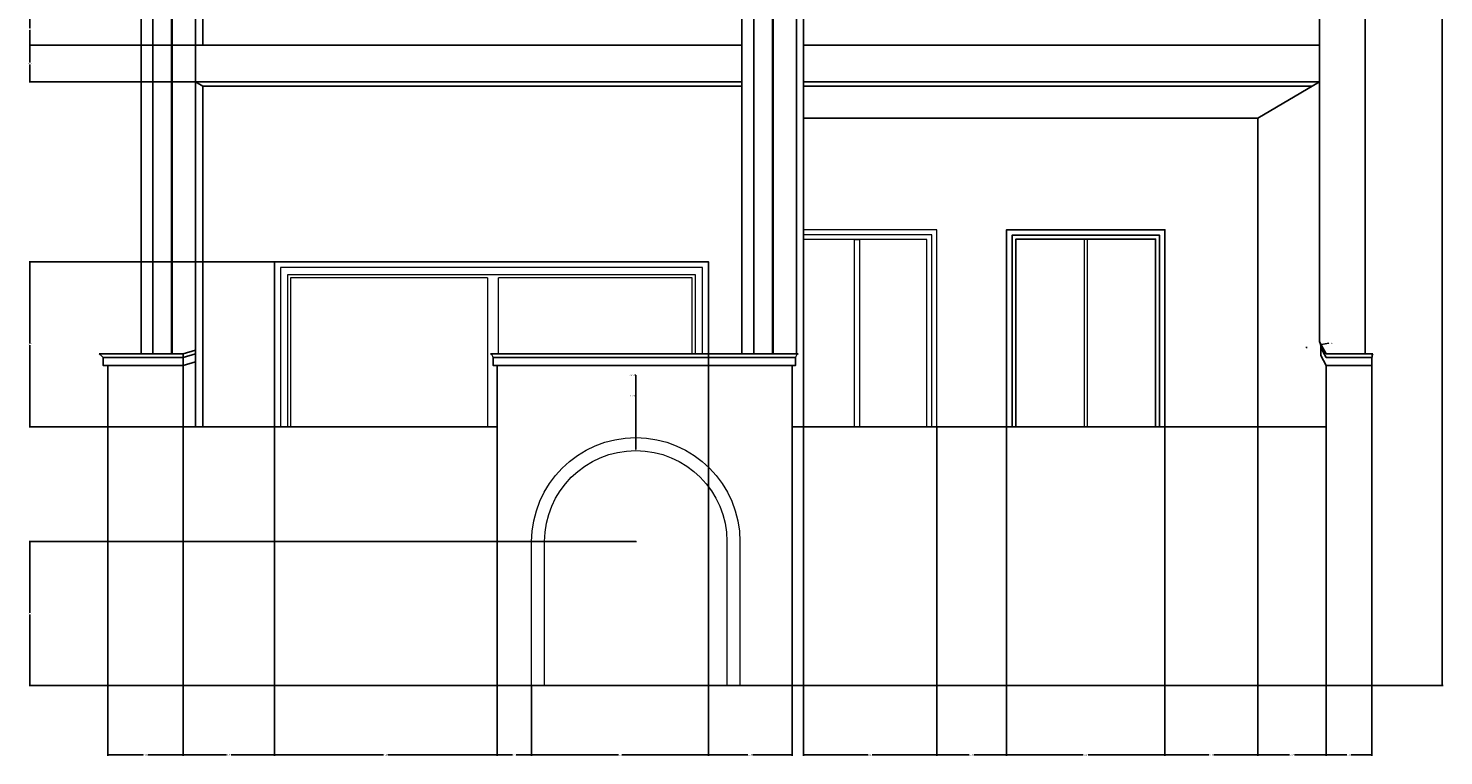
# Model space of a CAD drawing. Units: feet. Extents: x 2352 to 2983, y 950 to 1233.
# Tile 4 of 5: x 2718 to 2983, y 950 to 1086. Entities that reach past the tile are written whole.
import ezdxf

# ---------------------------------------------------------------- set-up
doc = ezdxf.new("R2010")
doc.units = ezdxf.units.FT
for name, color, linetype, lineweight in [('A-ANNO-DIMS', 2, 'Continuous', 18), ('A-DOOR', 3, 'Continuous', 18), ('A-ELEV', 7, 'Continuous', 25), ('A-GLAZ', 4, 'Continuous', 18)]:
    doc.layers.add(name, color=color, linetype=linetype, lineweight=lineweight)
doc.styles.get("Standard").update_dxf_attribs({"font": 'arial.ttf'})
doc.dimstyles.get("Standard").update_dxf_attribs({"dimtxt": 0.18, "dimasz": 0.18, "dimexe": 0.18, "dimexo": 0.0625, "dimgap": 0.09, "dimtad": 0, "dimtih": 1, "dimtoh": 1, "dimdec": 1, "dimzin": 0, "dimdsep": 46, "dimlunit": 3, "dimtxsty": 'Standard', "dimcen": 0.09, "dimadec": 0, "dimazin": 0, "dimtfac": 1, "dimtdec": 1, "dimtofl": 0, "dimtmove": 0, "dimatfit": 3, "dimfxl": 1, "dimtolj": 1, "dimtzin": 0, "dimarcsym": 0})

# ---------------------------------------------------------------- blocks, each defined once
blk = doc.blocks.new('*D30')
at = {"layer": 'A-ANNO-DIMS', "color": 0, "lineweight": -2, "transparency": 16777216}
for p, q in [((2934.99, 1219.82), (2982.56, 1219.82)), ((2982.38, 1219.64), (2982.38, 1091.6)), ((2982.38, 963.19), (2982.38, 1091.23)), ((2969.32, 963.01), (2982.56, 963.01))]:
    blk.add_line(p, q, dxfattribs=at)
at = {"layer": 'A-ANNO-DIMS', "color": 0, "transparency": 16777216}
for points in [[(2982.35, 1219.64), (2982.41, 1219.64), (2982.38, 1219.82)], [(2982.35, 963.19), (2982.41, 963.19), (2982.38, 963.01)]]:
    blk.add_solid(points, dxfattribs=at)
at = {"layer": 'Defpoints', "color": 0, "transparency": 16777216}
for p in [(2934.93, 1219.82), (2982.38, 1219.82), (2969.25, 963.01)]:
    blk.add_point(p, dxfattribs=at)
at = {"layer": 'A-ANNO-DIMS', "color": 0, "transparency": 16777216, "insert": (2982.38, 1091.42), "char_height": 0.18, "attachment_point": 5}
blk.add_mtext('\\A1;256.8', dxfattribs=at)
blk = doc.blocks.new('*D31')
at = {"layer": 'A-ANNO-DIMS', "color": 0, "lineweight": -2, "transparency": 16777216}
for p, q in [((2732.56, 962.95), (2732.56, 949.88)), ((2746.64, 962.95), (2746.64, 949.88)), ((2732.74, 950.06), (2739.15, 950.06)), ((2746.46, 950.06), (2740.06, 950.06))]:
    blk.add_line(p, q, dxfattribs=at)
at = {"layer": 'A-ANNO-DIMS', "color": 0, "transparency": 16777216}
for points in [[(2732.74, 950.09), (2732.74, 950.03), (2732.56, 950.06)], [(2746.46, 950.09), (2746.46, 950.03), (2746.64, 950.06)]]:
    blk.add_solid(points, dxfattribs=at)
at = {"layer": 'Defpoints', "color": 0, "transparency": 16777216}
for p in [(2732.56, 963.01), (2746.64, 963.01), (2746.64, 950.06)]:
    blk.add_point(p, dxfattribs=at)
at = {"layer": 'A-ANNO-DIMS', "color": 0, "transparency": 16777216, "insert": (2739.6, 950.06), "char_height": 0.18, "attachment_point": 5}
blk.add_mtext('\\A1;14.086', dxfattribs=at)
blk = doc.blocks.new('*D32')
at = {"layer": 'A-ANNO-DIMS', "color": 0, "lineweight": -2, "transparency": 16777216}
for p, q in [((2763.74, 1011.42), (2763.74, 949.88)), ((2746.64, 962.95), (2746.64, 949.88)), ((2746.82, 950.06), (2754.74, 950.06)), ((2763.56, 950.06), (2755.65, 950.06))]:
    blk.add_line(p, q, dxfattribs=at)
at = {"layer": 'A-ANNO-DIMS', "color": 0, "transparency": 16777216}
for points in [[(2746.82, 950.09), (2746.82, 950.03), (2746.64, 950.06)], [(2763.56, 950.09), (2763.56, 950.03), (2763.74, 950.06)]]:
    blk.add_solid(points, dxfattribs=at)
at = {"layer": 'Defpoints', "color": 0, "transparency": 16777216}
for p in [(2763.74, 1011.48), (2746.64, 963.01), (2763.74, 950.06)]:
    blk.add_point(p, dxfattribs=at)
at = {"layer": 'A-ANNO-DIMS', "color": 0, "transparency": 16777216, "insert": (2755.19, 950.06), "char_height": 0.18, "attachment_point": 5}
blk.add_mtext('\\A1;17.097', dxfattribs=at)
blk = doc.blocks.new('*D33')
at = {"layer": 'A-ANNO-DIMS', "color": 0, "lineweight": -2, "transparency": 16777216}
for p, q in [((2763.74, 1011.42), (2763.74, 949.88)), ((2805.43, 962.95), (2805.43, 949.88)), ((2763.92, 950.06), (2784.19, 950.06)), ((2805.25, 950.06), (2784.98, 950.06))]:
    blk.add_line(p, q, dxfattribs=at)
at = {"layer": 'A-ANNO-DIMS', "color": 0, "transparency": 16777216}
for points in [[(2763.92, 950.09), (2763.92, 950.03), (2763.74, 950.06)], [(2805.25, 950.09), (2805.25, 950.03), (2805.43, 950.06)]]:
    blk.add_solid(points, dxfattribs=at)
at = {"layer": 'Defpoints', "color": 0, "transparency": 16777216}
for p in [(2763.74, 1011.48), (2805.43, 963.01), (2805.43, 950.06)]:
    blk.add_point(p, dxfattribs=at)
at = {"layer": 'A-ANNO-DIMS', "color": 0, "transparency": 16777216, "insert": (2784.59, 950.06), "char_height": 0.18, "attachment_point": 5}
blk.add_mtext('\\A1;41.69', dxfattribs=at)
blk = doc.blocks.new('*D34')
at = {"layer": 'A-ANNO-DIMS', "color": 0, "lineweight": -2, "transparency": 16777216}
for p, q in [((2805.43, 962.95), (2805.43, 949.88)), ((2811.91, 962.95), (2811.91, 949.88)), ((2805.61, 950.06), (2808.35, 950.06)), ((2811.73, 950.06), (2809, 950.06))]:
    blk.add_line(p, q, dxfattribs=at)
at = {"layer": 'A-ANNO-DIMS', "color": 0, "transparency": 16777216}
for points in [[(2805.61, 950.09), (2805.61, 950.03), (2805.43, 950.06)], [(2811.73, 950.09), (2811.73, 950.03), (2811.91, 950.06)]]:
    blk.add_solid(points, dxfattribs=at)
at = {"layer": 'Defpoints', "color": 0, "transparency": 16777216}
for p in [(2805.43, 963.01), (2811.91, 963.01), (2811.91, 950.06)]:
    blk.add_point(p, dxfattribs=at)
at = {"layer": 'A-ANNO-DIMS', "color": 0, "transparency": 16777216, "insert": (2808.67, 950.06), "char_height": 0.18, "attachment_point": 5}
blk.add_mtext('\\A1;6.48', dxfattribs=at)
blk = doc.blocks.new('*D35')
at = {"layer": 'A-ANNO-DIMS', "color": 0, "lineweight": -2, "transparency": 16777216}
for p, q in [((2845.01, 1042.39), (2845.01, 949.88)), ((2811.91, 962.95), (2811.91, 949.88)), ((2812.09, 950.06), (2828.16, 950.06)), ((2844.83, 950.06), (2828.77, 950.06))]:
    blk.add_line(p, q, dxfattribs=at)
at = {"layer": 'A-ANNO-DIMS', "color": 0, "transparency": 16777216}
for points in [[(2812.09, 950.09), (2812.09, 950.03), (2811.91, 950.06)], [(2844.83, 950.09), (2844.83, 950.03), (2845.01, 950.06)]]:
    blk.add_solid(points, dxfattribs=at)
at = {"layer": 'Defpoints', "color": 0, "transparency": 16777216}
for p in [(2845.01, 1042.45), (2811.91, 963.01), (2845.01, 950.06)]:
    blk.add_point(p, dxfattribs=at)
at = {"layer": 'A-ANNO-DIMS', "color": 0, "transparency": 16777216, "insert": (2828.46, 950.06), "char_height": 0.18, "attachment_point": 5}
blk.add_mtext('\\A1;33.1', dxfattribs=at)
blk = doc.blocks.new('*D36')
at = {"layer": 'A-ANNO-DIMS', "color": 0, "lineweight": -2, "transparency": 16777216}
for p, q in [((2845.01, 1042.39), (2845.01, 949.88)), ((2860.71, 962.95), (2860.71, 949.88)), ((2845.19, 950.06), (2852.41, 950.06)), ((2860.53, 950.06), (2853.32, 950.06))]:
    blk.add_line(p, q, dxfattribs=at)
at = {"layer": 'A-ANNO-DIMS', "color": 0, "transparency": 16777216}
for points in [[(2845.19, 950.09), (2845.19, 950.03), (2845.01, 950.06)], [(2860.53, 950.09), (2860.53, 950.03), (2860.71, 950.06)]]:
    blk.add_solid(points, dxfattribs=at)
at = {"layer": 'Defpoints', "color": 0, "transparency": 16777216}
for p in [(2845.01, 1042.45), (2860.71, 963.01), (2860.71, 950.06)]:
    blk.add_point(p, dxfattribs=at)
at = {"layer": 'A-ANNO-DIMS', "color": 0, "transparency": 16777216, "insert": (2852.86, 950.06), "char_height": 0.18, "attachment_point": 5}
blk.add_mtext('\\A1;15.698', dxfattribs=at)
blk = doc.blocks.new('*D37')
at = {"layer": 'A-ANNO-DIMS', "color": 0, "lineweight": -2, "transparency": 16777216}
for p, q in [((2862.83, 1011.42), (2862.83, 949.88)), ((2887.78, 1011.42), (2887.78, 949.88)), ((2863.01, 950.06), (2874.91, 950.06)), ((2887.6, 950.06), (2875.7, 950.06))]:
    blk.add_line(p, q, dxfattribs=at)
at = {"layer": 'A-ANNO-DIMS', "color": 0, "transparency": 16777216}
for points in [[(2863.01, 950.09), (2863.01, 950.03), (2862.83, 950.06)], [(2887.6, 950.09), (2887.6, 950.03), (2887.78, 950.06)]]:
    blk.add_solid(points, dxfattribs=at)
at = {"layer": 'Defpoints', "color": 0, "transparency": 16777216}
for p in [(2862.83, 1011.48), (2887.78, 1011.48), (2887.78, 950.06)]:
    blk.add_point(p, dxfattribs=at)
at = {"layer": 'A-ANNO-DIMS', "color": 0, "transparency": 16777216, "insert": (2875.3, 950.06), "char_height": 0.18, "attachment_point": 5}
blk.add_mtext('\\A1;24.95', dxfattribs=at)
blk = doc.blocks.new('*D38')
at = {"layer": 'A-ANNO-DIMS', "color": 0, "lineweight": -2, "transparency": 16777216}
for p, q in [((2887.78, 1011.42), (2887.78, 949.88)), ((2900.84, 1011.42), (2900.84, 949.88)), ((2887.96, 950.06), (2893.85, 950.06)), ((2900.66, 950.06), (2894.76, 950.06))]:
    blk.add_line(p, q, dxfattribs=at)
at = {"layer": 'A-ANNO-DIMS', "color": 0, "transparency": 16777216}
for points in [[(2887.96, 950.09), (2887.96, 950.03), (2887.78, 950.06)], [(2900.66, 950.09), (2900.66, 950.03), (2900.84, 950.06)]]:
    blk.add_solid(points, dxfattribs=at)
at = {"layer": 'Defpoints', "color": 0, "transparency": 16777216}
for p in [(2887.78, 1011.48), (2900.84, 1011.48), (2900.84, 950.06)]:
    blk.add_point(p, dxfattribs=at)
at = {"layer": 'A-ANNO-DIMS', "color": 0, "transparency": 16777216, "insert": (2894.31, 950.06), "char_height": 0.18, "attachment_point": 5}
blk.add_mtext('\\A1;13.062', dxfattribs=at)
blk = doc.blocks.new('*D39')
at = {"layer": 'A-ANNO-DIMS', "color": 0, "lineweight": -2, "transparency": 16777216}
for p, q in [((2900.84, 1011.42), (2900.84, 949.88)), ((2930.49, 1011.42), (2930.49, 949.88)), ((2901.02, 950.06), (2915.2, 950.06)), ((2930.31, 950.06), (2916.13, 950.06))]:
    blk.add_line(p, q, dxfattribs=at)
at = {"layer": 'A-ANNO-DIMS', "color": 0, "transparency": 16777216}
for points in [[(2901.02, 950.09), (2901.02, 950.03), (2900.84, 950.06)], [(2930.31, 950.09), (2930.31, 950.03), (2930.49, 950.06)]]:
    blk.add_solid(points, dxfattribs=at)
at = {"layer": 'Defpoints', "color": 0, "transparency": 16777216}
for p in [(2900.84, 1011.48), (2930.49, 1011.48), (2930.49, 950.06)]:
    blk.add_point(p, dxfattribs=at)
at = {"layer": 'A-ANNO-DIMS', "color": 0, "transparency": 16777216, "insert": (2915.67, 950.06), "char_height": 0.18, "attachment_point": 5}
blk.add_mtext('\\A1;29.654', dxfattribs=at)
blk = doc.blocks.new('*D40')
at = {"layer": 'A-ANNO-DIMS', "color": 0, "lineweight": -2, "transparency": 16777216}
for p, q in [((2930.49, 1011.42), (2930.49, 949.88)), ((2947.9, 1011.42), (2947.9, 949.88)), ((2930.67, 950.06), (2938.74, 950.06)), ((2947.72, 950.06), (2939.65, 950.06))]:
    blk.add_line(p, q, dxfattribs=at)
at = {"layer": 'A-ANNO-DIMS', "color": 0, "transparency": 16777216}
for points in [[(2930.67, 950.09), (2930.67, 950.03), (2930.49, 950.06)], [(2947.72, 950.09), (2947.72, 950.03), (2947.9, 950.06)]]:
    blk.add_solid(points, dxfattribs=at)
at = {"layer": 'Defpoints', "color": 0, "transparency": 16777216}
for p in [(2930.49, 1011.48), (2947.9, 1011.48), (2947.9, 950.06)]:
    blk.add_point(p, dxfattribs=at)
at = {"layer": 'A-ANNO-DIMS', "color": 0, "transparency": 16777216, "insert": (2939.19, 950.06), "char_height": 0.18, "attachment_point": 5}
blk.add_mtext('\\A1;17.403', dxfattribs=at)
blk = doc.blocks.new('*D41')
at = {"layer": 'A-ANNO-DIMS', "color": 0, "lineweight": -2, "transparency": 16777216}
for p, q in [((2947.9, 1011.42), (2947.9, 949.88)), ((2960.69, 962.95), (2960.69, 949.88)), ((2948.08, 950.06), (2953.84, 950.06)), ((2960.51, 950.06), (2954.75, 950.06))]:
    blk.add_line(p, q, dxfattribs=at)
at = {"layer": 'A-ANNO-DIMS', "color": 0, "transparency": 16777216}
for points in [[(2948.08, 950.09), (2948.08, 950.03), (2947.9, 950.06)], [(2960.51, 950.09), (2960.51, 950.03), (2960.69, 950.06)]]:
    blk.add_solid(points, dxfattribs=at)
at = {"layer": 'Defpoints', "color": 0, "transparency": 16777216}
for p in [(2947.9, 1011.48), (2960.69, 963.01), (2960.69, 950.06)]:
    blk.add_point(p, dxfattribs=at)
at = {"layer": 'A-ANNO-DIMS', "color": 0, "transparency": 16777216, "insert": (2954.29, 950.06), "char_height": 0.18, "attachment_point": 5}
blk.add_mtext('\\A1;12.797', dxfattribs=at)
blk = doc.blocks.new('*D42')
at = {"layer": 'A-ANNO-DIMS', "color": 0, "lineweight": -2, "transparency": 16777216}
for p, q in [((2960.69, 962.95), (2960.69, 949.88)), ((2969.25, 962.95), (2969.25, 949.88)), ((2960.87, 950.06), (2964.58, 950.06)), ((2969.07, 950.06), (2965.37, 950.06))]:
    blk.add_line(p, q, dxfattribs=at)
at = {"layer": 'A-ANNO-DIMS', "color": 0, "transparency": 16777216}
for points in [[(2960.87, 950.09), (2960.87, 950.03), (2960.69, 950.06)], [(2969.07, 950.09), (2969.07, 950.03), (2969.25, 950.06)]]:
    blk.add_solid(points, dxfattribs=at)
at = {"layer": 'Defpoints', "color": 0, "transparency": 16777216}
for p in [(2960.69, 963.01), (2969.25, 963.01), (2969.25, 950.06)]:
    blk.add_point(p, dxfattribs=at)
at = {"layer": 'A-ANNO-DIMS', "color": 0, "transparency": 16777216, "insert": (2964.97, 950.06), "char_height": 0.18, "attachment_point": 5}
blk.add_mtext('\\A1;8.562', dxfattribs=at)
blk = doc.blocks.new('*D53')
at = {"layer": 'A-ANNO-DIMS', "color": 0, "lineweight": -2, "transparency": 16777216}
for p, q in [((2831.35, 989.99), (2717.79, 989.99)), ((2717.97, 989.81), (2717.97, 976.68)), ((2717.97, 963.19), (2717.97, 976.32)), ((2850.84, 963.01), (2717.79, 963.01))]:
    blk.add_line(p, q, dxfattribs=at)
at = {"layer": 'A-ANNO-DIMS', "color": 0, "transparency": 16777216}
for points in [[(2717.94, 989.81), (2718, 989.81), (2717.97, 989.99)], [(2717.94, 963.19), (2718, 963.19), (2717.97, 963.01)]]:
    blk.add_solid(points, dxfattribs=at)
at = {"layer": 'Defpoints', "color": 0, "transparency": 16777216}
for p in [(2717.97, 989.99), (2831.41, 989.99), (2850.91, 963.01)]:
    blk.add_point(p, dxfattribs=at)
at = {"layer": 'A-ANNO-DIMS', "color": 0, "transparency": 16777216, "insert": (2717.97, 976.5), "char_height": 0.18, "attachment_point": 5}
blk.add_mtext('\\A1;26.98', dxfattribs=at)
blk = doc.blocks.new('*D54')
at = {"layer": 'A-ANNO-DIMS', "color": 0, "lineweight": -2, "transparency": 16777216}
for p, q in [((2763.68, 1042.45), (2717.79, 1042.45)), ((2717.97, 1042.27), (2717.97, 1027.15)), ((2717.97, 1011.66), (2717.97, 1026.79)), ((2763.68, 1011.48), (2717.79, 1011.48))]:
    blk.add_line(p, q, dxfattribs=at)
at = {"layer": 'A-ANNO-DIMS', "color": 0, "transparency": 16777216}
for points in [[(2717.94, 1042.27), (2718, 1042.27), (2717.97, 1042.45)], [(2717.94, 1011.66), (2718, 1011.66), (2717.97, 1011.48)]]:
    blk.add_solid(points, dxfattribs=at)
at = {"layer": 'Defpoints', "color": 0, "transparency": 16777216}
for p in [(2717.97, 1042.45), (2763.74, 1042.45), (2763.74, 1011.48)]:
    blk.add_point(p, dxfattribs=at)
at = {"layer": 'A-ANNO-DIMS', "color": 0, "transparency": 16777216, "insert": (2717.97, 1026.97), "char_height": 0.18, "attachment_point": 5}
blk.add_mtext('\\A1;30.97', dxfattribs=at)
blk = doc.blocks.new('*D55')
at = {"layer": 'A-ANNO-DIMS', "color": 0, "lineweight": -2, "transparency": 16777216}
for p, q in [((2748.9, 1083.01), (2717.79, 1083.01)), ((2717.97, 1082.83), (2717.97, 1079.75)), ((2717.97, 1076.3), (2717.97, 1079.38)), ((2748.9, 1076.12), (2717.79, 1076.12))]:
    blk.add_line(p, q, dxfattribs=at)
at = {"layer": 'A-ANNO-DIMS', "color": 0, "transparency": 16777216}
for points in [[(2717.94, 1082.83), (2718, 1082.83), (2717.97, 1083.01)], [(2717.94, 1076.3), (2718, 1076.3), (2717.97, 1076.12)]]:
    blk.add_solid(points, dxfattribs=at)
at = {"layer": 'Defpoints', "color": 0, "transparency": 16777216}
for p in [(2717.97, 1083.01), (2748.96, 1083.01), (2748.96, 1076.12)]:
    blk.add_point(p, dxfattribs=at)
at = {"layer": 'A-ANNO-DIMS', "color": 0, "transparency": 16777216, "insert": (2717.97, 1079.57), "char_height": 0.18, "attachment_point": 5}
blk.add_mtext('\\A1;6.892', dxfattribs=at)
blk = doc.blocks.new('*D56')
at = {"layer": 'A-ANNO-DIMS', "color": 0, "lineweight": -2, "transparency": 16777216}
for p, q in [((2750.25, 1089.01), (2717.79, 1089.01)), ((2717.97, 1088.83), (2717.97, 1086.19)), ((2717.97, 1083.19), (2717.97, 1085.83)), ((2748.9, 1083.01), (2717.79, 1083.01))]:
    blk.add_line(p, q, dxfattribs=at)
at = {"layer": 'A-ANNO-DIMS', "color": 0, "transparency": 16777216}
for points in [[(2717.94, 1088.83), (2718, 1088.83), (2717.97, 1089.01)], [(2717.94, 1083.19), (2718, 1083.19), (2717.97, 1083.01)]]:
    blk.add_solid(points, dxfattribs=at)
at = {"layer": 'Defpoints', "color": 0, "transparency": 16777216}
for p in [(2717.97, 1089.01), (2750.31, 1089.01), (2748.96, 1083.01)]:
    blk.add_point(p, dxfattribs=at)
at = {"layer": 'A-ANNO-DIMS', "color": 0, "transparency": 16777216, "insert": (2717.97, 1086.01), "char_height": 0.18, "attachment_point": 5}
blk.add_mtext('\\A1;6', dxfattribs=at)
blk = doc.blocks.new('*D70')
at = {"layer": 'A-ANNO-DIMS', "color": 0, "lineweight": -2, "transparency": 16777216}
for p, q in [((2831.23, 1021.19), (2831.41, 1021.19)), ((2831.41, 1021.19), (2831.41, 1009.67)), ((2831.32, 989.99), (2831.5, 989.99)), ((2831.41, 989.9), (2831.41, 990.08))]:
    blk.add_line(p, q, dxfattribs=at)
at = {"layer": 'A-ANNO-DIMS', "color": 0, "transparency": 16777216}
blk.add_solid([(2831.44, 1009.67), (2831.38, 1009.67), (2831.41, 1009.49)], dxfattribs=at)
at = {"layer": 'Defpoints', "color": 0, "transparency": 16777216}
for p in [(2831.41, 1009.49), (2831.41, 989.99)]:
    blk.add_point(p, dxfattribs=at)
at = {"layer": 'A-ANNO-DIMS', "color": 0, "transparency": 16777216, "insert": (2830.68, 1021.19), "char_height": 0.18, "attachment_point": 5}
blk.add_mtext('\\A1;R19.497', dxfattribs=at)
blk = doc.blocks.new('*D71')
at = {"layer": 'A-ANNO-DIMS', "color": 0, "lineweight": -2, "transparency": 16777216}
for p, q in [((2831.23, 1017.31), (2831.41, 1017.31)), ((2831.41, 1017.31), (2831.41, 1007.24)), ((2831.32, 989.99), (2831.5, 989.99)), ((2831.41, 989.9), (2831.41, 990.08))]:
    blk.add_line(p, q, dxfattribs=at)
at = {"layer": 'A-ANNO-DIMS', "color": 0, "transparency": 16777216}
blk.add_solid([(2831.44, 1007.24), (2831.38, 1007.24), (2831.41, 1007.06)], dxfattribs=at)
at = {"layer": 'Defpoints', "color": 0, "transparency": 16777216}
for p in [(2831.41, 1007.06), (2831.41, 989.99)]:
    blk.add_point(p, dxfattribs=at)
at = {"layer": 'A-ANNO-DIMS', "color": 0, "transparency": 16777216, "insert": (2830.75, 1017.31), "char_height": 0.18, "attachment_point": 5}
blk.add_mtext('\\A1;R17.07', dxfattribs=at)
blk = doc.blocks.new('*D75')
at = {"layer": 'A-ANNO-DIMS', "color": 0, "lineweight": -2, "transparency": 16777216}
for p, q in [((2956.93, 1026.39), (2957.11, 1026.39)), ((2957.02, 1026.3), (2957.02, 1026.48)), ((2961.19, 1027.19), (2959.8, 1026.92))]:
    blk.add_line(p, q, dxfattribs=at)
at = {"layer": 'A-ANNO-DIMS', "color": 0, "transparency": 16777216}
blk.add_solid([(2959.8, 1026.95), (2959.81, 1026.89), (2959.63, 1026.89)], dxfattribs=at)
at = {"layer": 'Defpoints', "color": 0, "transparency": 16777216}
for p in [(2957.02, 1026.39), (2959.63, 1026.89)]:
    blk.add_point(p, dxfattribs=at)
at = {"layer": 'A-ANNO-DIMS', "color": 0, "transparency": 16777216, "insert": (2961.6, 1027.19), "char_height": 0.18, "attachment_point": 5}
blk.add_mtext('\\A1;R2.65', dxfattribs=at)

msp = doc.modelspace()

# ---------------------------------------------------------------- linework, layer by layer
at = {"layer": 'A-DOOR'}
for points in [[(2862.8263, 1011.4831), (2887.7768, 1011.4831), (2887.7768, 1048.4289), (2862.8263, 1048.4289)], [(2872.3434, 1046.5779), (2873.2689, 1046.5779), (2873.2689, 1011.4831), (2872.3434, 1011.4831)], [(2915.4169, 1046.6724), (2915.9141, 1046.6724), (2915.9141, 1011.4831), (2915.4169, 1011.4831)]]:
    msp.add_lwpolyline(points, close=True, dxfattribs=at)
for points in [[(2886.8407, 1011.4831), (2886.8407, 1047.4929), (2862.8263, 1047.4929)], [(2885.9258, 1011.4831), (2885.9258, 1046.5779), (2862.8263, 1046.5779)]]:
    msp.add_lwpolyline(points, dxfattribs=at)
msp.add_lwpolyline([(2850.9063, 989.9926), (2850.9063, 963.0126), (2811.9121, 963.0126), (2811.9121, 989.9926, -1)], format="xyb", close=True, dxfattribs=at)
msp.add_lwpolyline([(2814.3385, 963.0126), (2814.3385, 989.9926, -1), (2848.4799, 989.9926), (2848.4799, 963.0126)], format="xyb", dxfattribs=at)
msp.add_arc((2862.3432, 1024.3349), 1.0206, 120.460852, 171.077099, dxfattribs=at)
at = {"layer": 'A-ELEV'}
for p, q in [((2750.3114, 1083.0126), (2851.2955, 1083.0126)), ((2862.8263, 1083.0126), (2959.4504, 1083.0126)), ((2748.962, 1076.1207), (2750.3114, 1075.3288)), ((2947.8952, 1069.3398), (2959.4504, 1076.1207)), ((2750.3114, 1075.3288), (2851.2955, 1075.3288)), ((2862.8263, 1075.3288), (2958.101, 1075.3288)), ((2862.8263, 1069.3398), (2947.8952, 1069.3398)), ((2947.8952, 1069.3398), (2947.8952, 1011.4831)), ((2746.6445, 1025.2146), (2748.962, 1025.8769)), ((2748.962, 1011.4831), (2748.962, 1025.8769)), ((2960.6921, 1025.2146), (2959.4504, 1027.4578)), ((2960.6921, 1024.4932), (2959.6722, 1026.3357)), ((2959.6722, 1024.8551), (2959.6722, 1026.3357)), ((2746.6445, 1025.2146), (2730.9167, 1025.2146)), ((2732.5583, 963.0126), (2732.5583, 1023.0126)), ((2732.5583, 963.0126), (2732.5583, 1023.0126)), ((2746.6445, 1024.4932), (2746.6445, 1025.2146)), ((2746.6445, 1024.4932), (2748.962, 1025.1555)), ((2746.6445, 1023.0126), (2748.962, 1023.6749)), ((2861.8258, 1025.2146), (2804.2116, 1025.2146)), ((2960.6921, 1023.0126), (2959.6722, 1024.8551)), ((2969.2543, 1025.2146), (2960.6921, 1025.2146)), ((2969.2543, 1025.2146), (2969.429, 1025.2146)), ((2969.2543, 963.0126), (2969.2543, 1024.4932)), ((2732.5583, 963.0126), (2969.2543, 963.0126))]:
    msp.add_line(p, q, dxfattribs=at)
for points in [[(2959.4504, 1027.4578), (2959.4504, 1215.0126)], [(2968.0127, 1215.0126), (2968.0127, 1025.2146), (2960.6921, 1025.2146)], [(2862.8263, 1142.5724), (2862.8263, 1011.4831)], [(2738.7806, 1025.2146), (2738.7806, 1142.2389)], [(2750.3114, 1142.2389), (2750.3114, 1083.0126)], [(2851.2955, 1025.2146), (2851.2955, 1142.2389)], [(2853.4947, 1025.2146), (2853.4947, 1142.2389)], [(2861.477, 1142.2389), (2861.477, 1025.2146)], [(2740.9797, 1025.2146), (2740.9797, 1129.0147)], [(2744.4989, 1129.0147), (2744.4989, 1025.2146), (2744.5931, 1025.2146), (2744.5931, 1129.0147)], [(2748.962, 1129.0147), (2748.962, 1025.8769)], [(2857.0138, 1089.0126), (2857.0138, 1025.2146), (2857.108, 1025.2146), (2857.108, 1089.0126)], [(2750.3114, 1075.3288), (2750.3114, 1011.4831), (2746.6445, 1011.4831)], [(2901.8539, 1011.4831), (2901.8539, 1047.4133), (2929.4771, 1047.4133), (2929.4771, 1011.4831)], [(2902.5948, 1011.4831), (2902.5948, 1046.6724), (2928.7362, 1046.6724), (2928.7362, 1011.4831)], [(2845.0146, 1025.2146), (2845.0146, 1042.4514), (2763.7414, 1042.4514), (2763.7414, 1011.4831)], [(2960.6921, 1024.4932), (2969.2543, 1024.4932), (2969.2543, 1023.0126), (2960.6921, 1023.0126)]]:
    msp.add_lwpolyline(points, dxfattribs=at)
for points in [[(2748.962, 1083.0126), (2851.2955, 1083.0126), (2851.2955, 1076.1207), (2748.962, 1076.1207)], [(2862.8263, 1083.0126), (2959.4504, 1083.0126), (2959.4504, 1076.1207), (2862.8263, 1076.1207)], [(2930.4927, 1011.4831), (2900.8383, 1011.4831), (2900.8383, 1048.4289), (2930.4927, 1048.4289)], [(2731.6517, 1024.4932), (2746.6445, 1024.4932), (2746.6445, 1023.0126), (2731.6517, 1023.0126)], [(2732.5583, 963.0126), (2746.6445, 963.0126), (2746.6445, 1023.0126), (2732.5583, 1023.0126)], [(2804.7024, 1024.4932), (2861.335, 1024.4932), (2861.335, 1023.0126), (2804.7024, 1023.0126)], [(2805.432, 963.0126), (2860.7124, 963.0126), (2860.7124, 1023.0126), (2805.432, 1023.0126)], [(2960.6921, 963.0126), (2969.2543, 963.0126), (2969.2543, 1023.0126), (2960.6921, 1023.0126)], [(2746.6445, 963.0126), (2805.432, 963.0126), (2805.432, 1011.4831), (2746.6445, 1011.4831)], [(2860.7124, 963.0126), (2960.6921, 963.0126), (2960.6921, 1011.4831), (2860.7124, 1011.4831)]]:
    msp.add_lwpolyline(points, close=True, dxfattribs=at)
for centre, radius, start, end in [((2957.0223, 1026.3923), 2.6517, 357.9519, 23.693279), ((2729.8275, 1023.3696), 2.1425, 31.630035, 59.444961), ((2970.9987, 1024.4527), 1.7448, 154.108905, 178.670129)]:
    msp.add_arc(centre, radius, start, end, dxfattribs=at)
at = {"layer": 'A-GLAZ'}
for points in [[(2843.9015, 1025.2146), (2843.9015, 1041.3383), (2764.8545, 1041.3383), (2764.8545, 1011.4831)], [(2842.5736, 1025.2146), (2842.5736, 1040.0104), (2766.1823, 1040.0104), (2766.1823, 1011.4831)], [(2803.6699, 1039.4184), (2766.7743, 1039.4184), (2766.7743, 1011.4831)], [(2803.6699, 1039.4184), (2803.6699, 1011.4831)], [(2841.9816, 1025.2146), (2841.9816, 1039.4184), (2805.725, 1039.4184)], [(2805.725, 1025.2146), (2805.725, 1039.4184)]]:
    msp.add_lwpolyline(points, dxfattribs=at)
msp.add_arc((2803.6942, 1024.3349), 1.0206, 8.922901, 59.539148, dxfattribs=at)

# ---------------------------------------------------------------- dimensions: what is measured, and where the dimension line sits
at = {"layer": 'A-ANNO-DIMS'}
for base, p1, p2, override, picture, middle in [((2982.379, 1219.8182), (2969.2543, 963.0126), (2934.9257, 1219.8182), {"dimdec": 1, "dimlfac": 1, "dimrnd": 0, "dimzin": 0, "dimdsep": 46, "dimlunit": 2}, '*D30', (2982.379, 1091.4154)), ((2717.9667, 1089.0126), (2748.962, 1083.0126), (2750.3114, 1089.0126), {"dimdec": 0, "dimlfac": 1, "dimrnd": 0, "dimzin": 0, "dimdsep": 46, "dimlunit": 2}, '*D56', (2717.9667, 1086.0126)), ((2717.9667, 1083.0126), (2748.962, 1076.1207), (2748.962, 1083.0126), {"dimdec": 3, "dimlfac": 1, "dimrnd": 0, "dimzin": 0, "dimdsep": 46, "dimlunit": 2}, '*D55', (2717.9667, 1079.5667)), ((2717.9667, 1042.4514), (2763.7414, 1011.4831), (2763.7414, 1042.4514), {"dimdec": 2, "dimlfac": 1, "dimrnd": 0, "dimzin": 0, "dimdsep": 46, "dimlunit": 2}, '*D54', (2717.9667, 1026.9672)), ((2717.9667, 989.9926), (2850.9063, 963.0126), (2831.4092, 989.9926), {"dimdec": 2, "dimlfac": 1, "dimrnd": 0, "dimzin": 0, "dimdsep": 46, "dimlunit": 2}, '*D53', (2717.9667, 976.5026))]:
    dim = msp.add_linear_dim(base=base, p1=p1, p2=p2, angle=90, dimstyle='Standard', override=override, dxfattribs=at)
    dim.commit()
    dim.dimension.update_dxf_attribs({"geometry": picture, "text_midpoint": middle})
for base, p1, p2, override, picture, middle in [((2845.0146, 950.0626), (2811.9121, 963.0126), (2845.0146, 1042.4514), {"dimdec": 1, "dimlfac": 1, "dimrnd": 0, "dimzin": 0, "dimdsep": 46, "dimlunit": 2}, '*D35', (2828.4633, 950.0626)), ((2860.7124, 950.0626), (2845.0146, 1042.4514), (2860.7124, 963.0126), {"dimdec": 3, "dimlfac": 1, "dimrnd": 0, "dimzin": 0, "dimdsep": 46, "dimlunit": 2}, '*D36', (2852.8635, 950.0626)), ((2763.7414, 950.0626), (2746.6445, 963.0126), (2763.7414, 1011.4831), {"dimdec": 3, "dimlfac": 1, "dimrnd": 0, "dimzin": 0, "dimdsep": 46, "dimlunit": 2}, '*D32', (2755.1929, 950.0626)), ((2805.432, 950.0626), (2763.7414, 1011.4831), (2805.432, 963.0126), {"dimdec": 2, "dimlfac": 1, "dimrnd": 0, "dimzin": 0, "dimdsep": 46, "dimlunit": 2}, '*D33', (2784.5867, 950.0626)), ((2887.7768, 950.0626), (2862.8263, 1011.4831), (2887.7768, 1011.4831), {"dimdec": 2, "dimlfac": 1, "dimrnd": 0, "dimzin": 0, "dimdsep": 46, "dimlunit": 2}, '*D37', (2875.3016, 950.0626)), ((2900.83833, 950.06265), (2887.77675, 1011.48306), (2900.83833, 1011.48306), {"dimdec": 3, "dimlfac": 1, "dimrnd": 0, "dimzin": 0, "dimdsep": 46, "dimlunit": 2}, '*D38', (2894.30754, 950.06265)), ((2930.4927, 950.0626), (2900.8383, 1011.4831), (2930.4927, 1011.4831), {"dimdec": 3, "dimlfac": 1, "dimrnd": 0, "dimzin": 0, "dimdsep": 46, "dimlunit": 2}, '*D39', (2915.6655, 950.0626)), ((2947.89522, 950.06265), (2930.49267, 1011.48306), (2947.89522, 1011.48306), {"dimdec": 3, "dimlfac": 1, "dimrnd": 0, "dimzin": 0, "dimdsep": 46, "dimlunit": 2}, '*D40', (2939.19394, 950.06265)), ((2960.6921, 950.0626), (2947.8952, 1011.4831), (2960.6921, 963.0126), {"dimdec": 3, "dimlfac": 1, "dimrnd": 0, "dimzin": 0, "dimdsep": 46, "dimlunit": 2}, '*D41', (2954.2936, 950.0626)), ((2746.6445, 950.0626), (2732.5583, 963.0126), (2746.6445, 963.0126), {"dimdec": 3, "dimlfac": 1, "dimrnd": 0, "dimzin": 0, "dimdsep": 46, "dimlunit": 2}, '*D31', (2739.6014, 950.0626)), ((2811.9121, 950.0626), (2805.432, 963.0126), (2811.9121, 963.0126), {"dimdec": 2, "dimlfac": 1, "dimrnd": 0, "dimzin": 0, "dimdsep": 46, "dimlunit": 2}, '*D34', (2808.6721, 950.0626)), ((2969.2543, 950.0626), (2960.6921, 963.0126), (2969.2543, 963.0126), {"dimdec": 3, "dimlfac": 1, "dimrnd": 0, "dimzin": 0, "dimdsep": 46, "dimlunit": 2}, '*D42', (2964.9732, 950.0626))]:
    dim = msp.add_linear_dim(base=base, p1=p1, p2=p2, dimstyle='Standard', override=override, dxfattribs=at)
    dim.commit()
    dim.dimension.update_dxf_attribs({"geometry": picture, "text_midpoint": middle})
for center, mpoint, override, picture, middle in [((2957.0223, 1026.3923), (2959.6268, 1026.89), {"dimdec": 2, "dimlfac": 1, "dimrnd": 0, "dimzin": 0, "dimdsep": 46, "dimlunit": 2}, '*D75', (2961.1895, 1027.1886)), ((2831.4092, 989.9926), (2831.409, 1009.4897), {"dimdec": 3, "dimlfac": 1, "dimrnd": 0, "dimzin": 0, "dimdsep": 46, "dimlunit": 2}, '*D70', (2830.6791, 1021.188)), ((2831.4092, 989.9926), (2831.409, 1007.0633), {"dimdec": 2, "dimlfac": 1, "dimrnd": 0, "dimzin": 0, "dimdsep": 46, "dimlunit": 2}, '*D71', (2830.749, 1017.3057))]:
    dim = msp.add_radius_dim(center=center, mpoint=mpoint, dimstyle='Standard', override=override, dxfattribs=at)
    dim.commit()
    dim.dimension.update_dxf_attribs({"geometry": picture, "text_midpoint": middle, "dimtype": 164})

doc.saveas('drawing.dxf')
